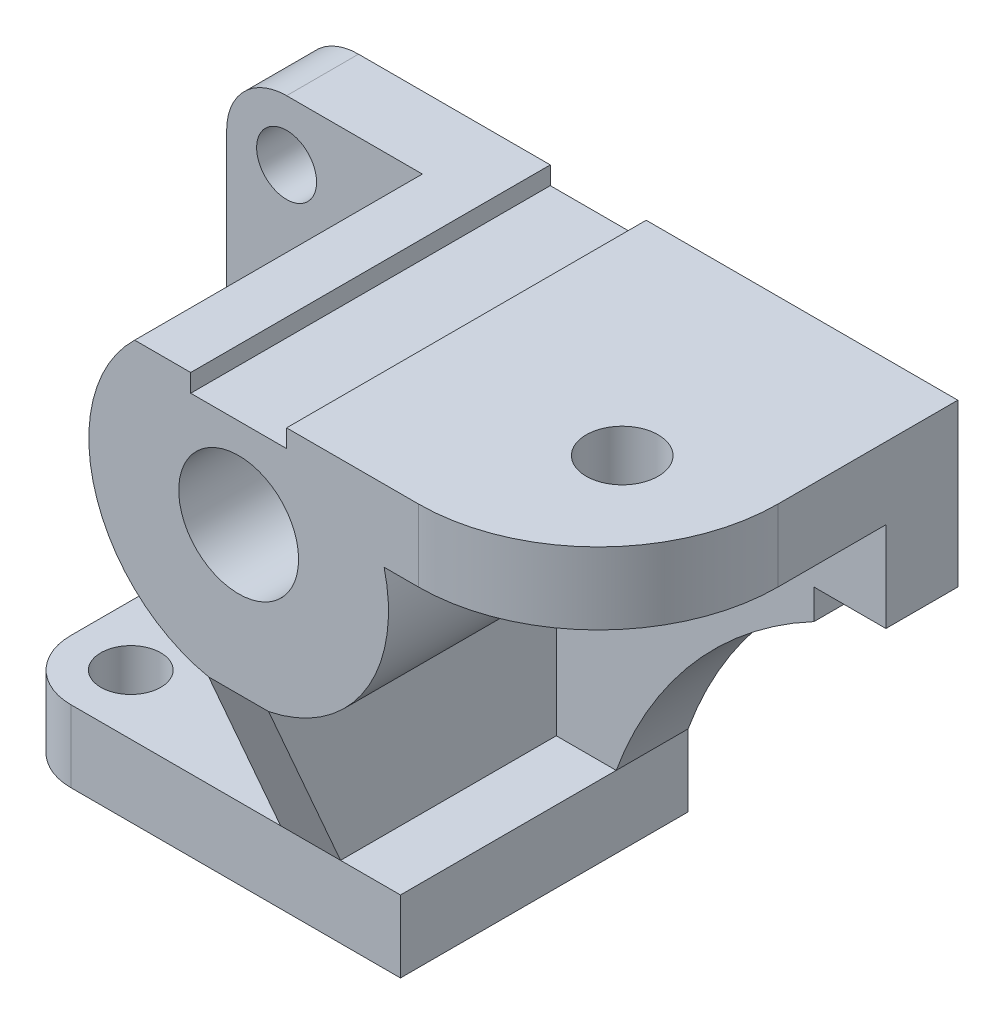
ISO-10303-21;
HEADER;
FILE_DESCRIPTION(('STEP AP214'),'2;1');
FILE_NAME('part.step','',(''),(''),'','','');
FILE_SCHEMA(('AUTOMOTIVE_DESIGN { 1 0 10303 214 1 1 1 1 }'));
ENDSEC;
DATA;
#1=APPLICATION_CONTEXT('core data for automotive mechanical design processes');
#2=APPLICATION_PROTOCOL_DEFINITION('international standard','automotive_design',2000,#1);
#3=PRODUCT_CONTEXT('',#1,'mechanical');
#4=PRODUCT('Part','Part','',(#3));
#5=PRODUCT_RELATED_PRODUCT_CATEGORY('part','',(#4));
#6=PRODUCT_DEFINITION_FORMATION('','',#4);
#7=PRODUCT_DEFINITION_CONTEXT('part definition',#1,'design');
#8=PRODUCT_DEFINITION('design','',#6,#7);
#9=PRODUCT_DEFINITION_SHAPE('','',#8);
#10=(LENGTH_UNIT() NAMED_UNIT(*) SI_UNIT(.MILLI.,.METRE.));
#11=(NAMED_UNIT(*) PLANE_ANGLE_UNIT() SI_UNIT($,.RADIAN.));
#12=(NAMED_UNIT(*) SI_UNIT($,.STERADIAN.) SOLID_ANGLE_UNIT());
#13=UNCERTAINTY_MEASURE_WITH_UNIT(LENGTH_MEASURE(1.E-05),#10,'distance_accuracy_value','');
#14=(GEOMETRIC_REPRESENTATION_CONTEXT(3) GLOBAL_UNCERTAINTY_ASSIGNED_CONTEXT((#13)) GLOBAL_UNIT_ASSIGNED_CONTEXT((#10,
#11,#12)) REPRESENTATION_CONTEXT('',''));
#15=CARTESIAN_POINT('',(0.,0.,0.));
#16=DIRECTION('',(0.,0.,1.));
#17=DIRECTION('',(1.,0.,0.));
#18=AXIS2_PLACEMENT_3D('',#15,#16,#17);
#19=CARTESIAN_POINT('',(98.3190383965627,-11.8296912391202,-12.));
#20=DIRECTION('',(0.,0.,1.));
#21=DIRECTION('',(1.,0.,0.));
#22=AXIS2_PLACEMENT_3D('',#19,#20,#21);
#23=PLANE('',#22);
#24=CARTESIAN_POINT('',(17.5,64.,-12.));
#25=DIRECTION('',(0.,0.,1.));
#26=DIRECTION('',(1.,0.,0.));
#27=AXIS2_PLACEMENT_3D('',#24,#25,#26);
#28=CIRCLE('',#27,25.);
#29=CARTESIAN_POINT('',(22.5,39.5051025721682,-12.));
#30=VERTEX_POINT('',#29);
#31=CARTESIAN_POINT('',(41.7693221990232,70.,-12.));
#32=VERTEX_POINT('',#31);
#33=EDGE_CURVE('E344',#30,#32,#28,.T.);
#34=ORIENTED_EDGE('',*,*,#33,.F.);
#35=DIRECTION('',(0.,1.,0.));
#36=VECTOR('',#35,1.);
#37=CARTESIAN_POINT('',(22.5,39.5051025721682,-12.));
#38=LINE('',#37,#36);
#39=CARTESIAN_POINT('',(22.5,12.,-12.));
#40=VERTEX_POINT('',#39);
#41=EDGE_CURVE('E428',#40,#30,#38,.T.);
#42=ORIENTED_EDGE('',*,*,#41,.F.);
#43=DIRECTION('',(-1.,0.,0.));
#44=VECTOR('',#43,1.);
#45=CARTESIAN_POINT('',(32.5,12.,-12.));
#46=LINE('',#45,#44);
#47=CARTESIAN_POINT('',(32.5,12.,-12.));
#48=VERTEX_POINT('',#47);
#49=EDGE_CURVE('E233',#48,#40,#46,.T.);
#50=ORIENTED_EDGE('',*,*,#49,.F.);
#51=CARTESIAN_POINT('',(98.3190383965627,-11.8296912391202,-12.));
#52=DIRECTION('',(0.,0.,1.));
#53=DIRECTION('',(1.,0.,0.));
#54=AXIS2_PLACEMENT_3D('',#51,#52,#53);
#55=CIRCLE('',#54,70.);
#56=CARTESIAN_POINT('',(65.5,50.,-12.));
#57=VERTEX_POINT('',#56);
#58=EDGE_CURVE('E377',#57,#48,#55,.T.);
#59=ORIENTED_EDGE('',*,*,#58,.F.);
#60=DIRECTION('',(0.,-1.,0.));
#61=VECTOR('',#60,1.);
#62=CARTESIAN_POINT('',(65.5,55.,-12.));
#63=LINE('',#62,#61);
#64=CARTESIAN_POINT('',(65.5,55.,-12.));
#65=VERTEX_POINT('',#64);
#66=EDGE_CURVE('E374',#65,#57,#63,.T.);
#67=ORIENTED_EDGE('',*,*,#66,.F.);
#68=DIRECTION('',(-1.,0.,0.));
#69=VECTOR('',#68,1.);
#70=CARTESIAN_POINT('',(77.5,55.,-12.));
#71=LINE('',#70,#69);
#72=CARTESIAN_POINT('',(77.5,55.,-12.));
#73=VERTEX_POINT('',#72);
#74=EDGE_CURVE('E375',#73,#65,#71,.T.);
#75=ORIENTED_EDGE('',*,*,#74,.F.);
#76=DIRECTION('',(0.,-1.,0.));
#77=VECTOR('',#76,1.);
#78=CARTESIAN_POINT('',(77.5,82.,-12.));
#79=LINE('',#78,#77);
#80=CARTESIAN_POINT('',(77.5,70.,-12.));
#81=VERTEX_POINT('',#80);
#82=EDGE_CURVE('E369',#81,#73,#79,.T.);
#83=ORIENTED_EDGE('',*,*,#82,.F.);
#84=DIRECTION('',(-1.,0.,0.));
#85=VECTOR('',#84,1.);
#86=CARTESIAN_POINT('',(98.3190383965627,70.,-12.));
#87=LINE('',#86,#85);
#88=EDGE_CURVE('E463',#81,#32,#87,.T.);
#89=ORIENTED_EDGE('',*,*,#88,.T.);
#90=EDGE_LOOP('',(#34,#42,#50,#59,#67,#75,#83,#89));
#91=FACE_BOUND('',#90,.T.);
#92=ADVANCED_FACE('F44',(#91),#23,.T.);
#93=CARTESIAN_POINT('',(-22.5,72.,-12.));
#94=DIRECTION('',(0.,0.,1.));
#95=DIRECTION('',(1.,0.,0.));
#96=AXIS2_PLACEMENT_3D('',#93,#94,#95);
#97=CIRCLE('',#96,5.);
#98=CARTESIAN_POINT('',(-17.5,72.,-12.));
#99=VERTEX_POINT('',#98);
#100=EDGE_CURVE('E441',#99,#99,#97,.T.);
#101=ORIENTED_EDGE('',*,*,#100,.F.);
#102=EDGE_LOOP('',(#101));
#103=FACE_BOUND('',#102,.T.);
#104=CARTESIAN_POINT('',(12.5,12.,-12.));
#105=VERTEX_POINT('',#104);
#106=CARTESIAN_POINT('',(-32.5,12.,-12.));
#107=VERTEX_POINT('',#106);
#108=EDGE_CURVE('E370',#105,#107,#46,.T.);
#109=ORIENTED_EDGE('',*,*,#108,.F.);
#110=DIRECTION('',(0.,-1.,0.));
#111=VECTOR('',#110,1.);
#112=CARTESIAN_POINT('',(12.5,12.,-12.));
#113=LINE('',#112,#111);
#114=CARTESIAN_POINT('',(12.5,39.5051025721682,-12.));
#115=VERTEX_POINT('',#114);
#116=EDGE_CURVE('E426',#115,#105,#113,.T.);
#117=ORIENTED_EDGE('',*,*,#116,.F.);
#118=CARTESIAN_POINT('',(0.150648427102509,82.,-12.));
#119=VERTEX_POINT('',#118);
#120=EDGE_CURVE('E349',#119,#115,#28,.T.);
#121=ORIENTED_EDGE('',*,*,#120,.F.);
#122=DIRECTION('',(1.,0.,0.));
#123=VECTOR('',#122,1.);
#124=CARTESIAN_POINT('',(-32.5,82.,-12.));
#125=LINE('',#124,#123);
#126=CARTESIAN_POINT('',(-22.5,82.,-12.));
#127=VERTEX_POINT('',#126);
#128=EDGE_CURVE('E292',#127,#119,#125,.T.);
#129=ORIENTED_EDGE('',*,*,#128,.F.);
#130=CARTESIAN_POINT('',(-22.5,72.,-12.));
#131=DIRECTION('',(0.,0.,1.));
#132=DIRECTION('',(1.,0.,0.));
#133=AXIS2_PLACEMENT_3D('',#130,#131,#132);
#134=CIRCLE('',#133,10.);
#135=CARTESIAN_POINT('',(-32.5,72.,-12.));
#136=VERTEX_POINT('',#135);
#137=EDGE_CURVE('E52',#127,#136,#134,.T.);
#138=ORIENTED_EDGE('',*,*,#137,.T.);
#139=DIRECTION('',(0.,1.,0.));
#140=VECTOR('',#139,1.);
#141=CARTESIAN_POINT('',(-32.5,12.,-12.));
#142=LINE('',#141,#140);
#143=EDGE_CURVE('E287',#107,#136,#142,.T.);
#144=ORIENTED_EDGE('',*,*,#143,.F.);
#145=EDGE_LOOP('',(#109,#117,#121,#129,#138,#144));
#146=FACE_BOUND('',#145,.T.);
#147=ADVANCED_FACE('F288',(#103,#146),#23,.T.);
#148=CARTESIAN_POINT('',(17.5,64.,36.));
#149=DIRECTION('',(0.,0.,-1.));
#150=DIRECTION('',(-1.,0.,0.));
#151=AXIS2_PLACEMENT_3D('',#148,#149,#150);
#152=CYLINDRICAL_SURFACE('',#151,25.);
#153=DIRECTION('',(0.,0.,-1.));
#154=VECTOR('',#153,1.);
#155=CARTESIAN_POINT('',(22.5,39.5051025721682,36.));
#156=LINE('',#155,#154);
#157=CARTESIAN_POINT('',(22.5,39.5051025721682,36.));
#158=VERTEX_POINT('',#157);
#159=EDGE_CURVE('E225',#158,#30,#156,.T.);
#160=ORIENTED_EDGE('',*,*,#159,.T.);
#161=ORIENTED_EDGE('',*,*,#33,.T.);
#162=DIRECTION('',(0.,0.,-1.));
#163=VECTOR('',#162,1.);
#164=CARTESIAN_POINT('',(41.7693221990232,70.,36.));
#165=LINE('',#164,#163);
#166=CARTESIAN_POINT('',(41.7693221990232,70.,36.));
#167=VERTEX_POINT('',#166);
#168=EDGE_CURVE('E457',#167,#32,#165,.T.);
#169=ORIENTED_EDGE('',*,*,#168,.F.);
#170=CARTESIAN_POINT('',(17.5,64.,36.));
#171=DIRECTION('',(0.,0.,1.));
#172=DIRECTION('',(1.,0.,0.));
#173=AXIS2_PLACEMENT_3D('',#170,#171,#172);
#174=CIRCLE('',#173,25.);
#175=EDGE_CURVE('E360',#158,#167,#174,.T.);
#176=ORIENTED_EDGE('',*,*,#175,.F.);
#177=EDGE_LOOP('',(#160,#161,#169,#176));
#178=FACE_BOUND('',#177,.T.);
#179=ADVANCED_FACE('F317',(#178),#152,.T.);
#180=DIRECTION('',(0.,0.,-1.));
#181=VECTOR('',#180,1.);
#182=CARTESIAN_POINT('',(12.5,39.5051025721682,36.));
#183=LINE('',#182,#181);
#184=CARTESIAN_POINT('',(12.5,39.5051025721682,36.));
#185=VERTEX_POINT('',#184);
#186=EDGE_CURVE('E434',#185,#115,#183,.T.);
#187=ORIENTED_EDGE('',*,*,#186,.F.);
#188=CARTESIAN_POINT('',(0.150648427102509,82.,36.));
#189=VERTEX_POINT('',#188);
#190=EDGE_CURVE('E354',#189,#185,#174,.T.);
#191=ORIENTED_EDGE('',*,*,#190,.F.);
#192=DIRECTION('',(0.,0.,-1.));
#193=VECTOR('',#192,1.);
#194=CARTESIAN_POINT('',(0.150648427102509,82.,36.));
#195=LINE('',#194,#193);
#196=EDGE_CURVE('E363',#189,#119,#195,.T.);
#197=ORIENTED_EDGE('',*,*,#196,.T.);
#198=ORIENTED_EDGE('',*,*,#120,.T.);
#199=EDGE_LOOP('',(#187,#191,#197,#198));
#200=FACE_BOUND('',#199,.T.);
#201=ADVANCED_FACE('F500',(#200),#152,.T.);
#202=CARTESIAN_POINT('',(0.,12.,0.));
#203=DIRECTION('',(0.,-1.,0.));
#204=DIRECTION('',(0.,0.,-1.));
#205=AXIS2_PLACEMENT_3D('',#202,#203,#204);
#206=PLANE('',#205);
#207=DIRECTION('',(0.,0.,-1.));
#208=VECTOR('',#207,1.);
#209=CARTESIAN_POINT('',(22.5,12.,36.));
#210=LINE('',#209,#208);
#211=CARTESIAN_POINT('',(22.5,12.,24.));
#212=VERTEX_POINT('',#211);
#213=EDGE_CURVE('E218',#212,#40,#210,.T.);
#214=ORIENTED_EDGE('',*,*,#213,.F.);
#215=DIRECTION('',(1.,0.,0.));
#216=VECTOR('',#215,1.);
#217=CARTESIAN_POINT('',(-32.5,12.,24.));
#218=LINE('',#217,#216);
#219=CARTESIAN_POINT('',(32.5,12.,24.));
#220=VERTEX_POINT('',#219);
#221=EDGE_CURVE('E214',#212,#220,#218,.T.);
#222=ORIENTED_EDGE('',*,*,#221,.T.);
#223=DIRECTION('',(0.,0.,-1.));
#224=VECTOR('',#223,1.);
#225=CARTESIAN_POINT('',(32.5,12.,24.));
#226=LINE('',#225,#224);
#227=EDGE_CURVE('E239',#220,#48,#226,.T.);
#228=ORIENTED_EDGE('',*,*,#227,.T.);
#229=ORIENTED_EDGE('',*,*,#49,.T.);
#230=EDGE_LOOP('',(#214,#222,#228,#229));
#231=FACE_BOUND('',#230,.T.);
#232=ADVANCED_FACE('F226',(#231),#206,.F.);
#233=CARTESIAN_POINT('',(-22.5,12.,14.));
#234=DIRECTION('',(0.,1.,0.));
#235=DIRECTION('',(0.,0.,1.));
#236=AXIS2_PLACEMENT_3D('',#233,#234,#235);
#237=CIRCLE('',#236,5.);
#238=CARTESIAN_POINT('',(-22.5,12.,19.));
#239=VERTEX_POINT('',#238);
#240=EDGE_CURVE('E235',#239,#239,#237,.T.);
#241=ORIENTED_EDGE('',*,*,#240,.F.);
#242=EDGE_LOOP('',(#241));
#243=FACE_BOUND('',#242,.T.);
#244=DIRECTION('',(0.,0.,-1.));
#245=VECTOR('',#244,1.);
#246=CARTESIAN_POINT('',(12.5,12.,36.));
#247=LINE('',#246,#245);
#248=CARTESIAN_POINT('',(12.5,12.,24.));
#249=VERTEX_POINT('',#248);
#250=EDGE_CURVE('E427',#249,#105,#247,.T.);
#251=ORIENTED_EDGE('',*,*,#250,.T.);
#252=ORIENTED_EDGE('',*,*,#108,.T.);
#253=DIRECTION('',(0.,0.,1.));
#254=VECTOR('',#253,1.);
#255=CARTESIAN_POINT('',(-32.5,12.,24.));
#256=LINE('',#255,#254);
#257=CARTESIAN_POINT('',(-32.5,12.,14.));
#258=VERTEX_POINT('',#257);
#259=EDGE_CURVE('E238',#107,#258,#256,.T.);
#260=ORIENTED_EDGE('',*,*,#259,.T.);
#261=CARTESIAN_POINT('',(-22.5,12.,14.));
#262=DIRECTION('',(0.,-1.,0.));
#263=DIRECTION('',(0.,0.,-1.));
#264=AXIS2_PLACEMENT_3D('',#261,#262,#263);
#265=CIRCLE('',#264,10.);
#266=CARTESIAN_POINT('',(-22.5,12.,24.));
#267=VERTEX_POINT('',#266);
#268=EDGE_CURVE('E278',#258,#267,#265,.F.);
#269=ORIENTED_EDGE('',*,*,#268,.T.);
#270=EDGE_CURVE('E215',#267,#249,#218,.T.);
#271=ORIENTED_EDGE('',*,*,#270,.T.);
#272=EDGE_LOOP('',(#251,#252,#260,#269,#271));
#273=FACE_BOUND('',#272,.T.);
#274=ADVANCED_FACE('F501',(#243,#273),#206,.F.);
#275=CARTESIAN_POINT('',(-32.5,82.,-12.));
#276=DIRECTION('',(0.,1.,0.));
#277=DIRECTION('',(0.,0.,1.));
#278=AXIS2_PLACEMENT_3D('',#275,#276,#277);
#279=PLANE('',#278);
#280=DIRECTION('',(1.,0.,0.));
#281=VECTOR('',#280,1.);
#282=CARTESIAN_POINT('',(-32.5,82.,-24.));
#283=LINE('',#282,#281);
#284=CARTESIAN_POINT('',(-22.5,82.,-24.));
#285=VERTEX_POINT('',#284);
#286=CARTESIAN_POINT('',(9.49999999999999,82.,-24.));
#287=VERTEX_POINT('',#286);
#288=EDGE_CURVE('E385',#285,#287,#283,.T.);
#289=ORIENTED_EDGE('',*,*,#288,.F.);
#290=DIRECTION('',(0.,0.,-1.));
#291=VECTOR('',#290,1.);
#292=CARTESIAN_POINT('',(-22.5,82.,-12.));
#293=LINE('',#292,#291);
#294=EDGE_CURVE('E58',#285,#127,#293,.F.);
#295=ORIENTED_EDGE('',*,*,#294,.T.);
#296=ORIENTED_EDGE('',*,*,#128,.T.);
#297=ORIENTED_EDGE('',*,*,#196,.F.);
#298=DIRECTION('',(-1.,0.,0.));
#299=VECTOR('',#298,1.);
#300=CARTESIAN_POINT('',(0.150648427102509,82.,36.));
#301=LINE('',#300,#299);
#302=CARTESIAN_POINT('',(9.49999999999999,82.,36.));
#303=VERTEX_POINT('',#302);
#304=EDGE_CURVE('E356',#303,#189,#301,.T.);
#305=ORIENTED_EDGE('',*,*,#304,.F.);
#306=DIRECTION('',(0.,0.,1.));
#307=VECTOR('',#306,1.);
#308=CARTESIAN_POINT('',(9.49999999999999,82.,-24.));
#309=LINE('',#308,#307);
#310=EDGE_CURVE('E464',#287,#303,#309,.T.);
#311=ORIENTED_EDGE('',*,*,#310,.F.);
#312=EDGE_LOOP('',(#289,#295,#296,#297,#305,#311));
#313=FACE_BOUND('',#312,.T.);
#314=ADVANCED_FACE('F491',(#313),#279,.T.);
#315=CARTESIAN_POINT('',(32.5,12.,24.));
#316=DIRECTION('',(-1.,0.,0.));
#317=DIRECTION('',(0.,0.,1.));
#318=AXIS2_PLACEMENT_3D('',#315,#316,#317);
#319=PLANE('',#318);
#320=DIRECTION('',(0.,0.,-1.));
#321=VECTOR('',#320,1.);
#322=CARTESIAN_POINT('',(32.5,0.,24.));
#323=LINE('',#322,#321);
#324=CARTESIAN_POINT('',(32.5,0.,24.));
#325=VERTEX_POINT('',#324);
#326=CARTESIAN_POINT('',(32.5,0.,-24.));
#327=VERTEX_POINT('',#326);
#328=EDGE_CURVE('E400',#325,#327,#323,.T.);
#329=ORIENTED_EDGE('',*,*,#328,.T.);
#330=DIRECTION('',(0.,-1.,0.));
#331=VECTOR('',#330,1.);
#332=CARTESIAN_POINT('',(32.5,12.,-24.));
#333=LINE('',#332,#331);
#334=CARTESIAN_POINT('',(32.5,12.,-24.));
#335=VERTEX_POINT('',#334);
#336=EDGE_CURVE('E249',#335,#327,#333,.T.);
#337=ORIENTED_EDGE('',*,*,#336,.F.);
#338=DIRECTION('',(0.,0.,-1.));
#339=VECTOR('',#338,1.);
#340=CARTESIAN_POINT('',(32.5,12.,-12.));
#341=LINE('',#340,#339);
#342=EDGE_CURVE('E392',#48,#335,#341,.T.);
#343=ORIENTED_EDGE('',*,*,#342,.F.);
#344=ORIENTED_EDGE('',*,*,#227,.F.);
#345=DIRECTION('',(0.,-1.,0.));
#346=VECTOR('',#345,1.);
#347=CARTESIAN_POINT('',(32.5,12.,24.));
#348=LINE('',#347,#346);
#349=EDGE_CURVE('E236',#220,#325,#348,.T.);
#350=ORIENTED_EDGE('',*,*,#349,.T.);
#351=EDGE_LOOP('',(#329,#337,#343,#344,#350));
#352=FACE_BOUND('',#351,.T.);
#353=ADVANCED_FACE('F413',(#352),#319,.F.);
#354=CARTESIAN_POINT('',(-32.5,12.,-24.));
#355=DIRECTION('',(0.,0.,1.));
#356=DIRECTION('',(1.,0.,0.));
#357=AXIS2_PLACEMENT_3D('',#354,#355,#356);
#358=PLANE('',#357);
#359=CARTESIAN_POINT('',(-22.5,72.,-24.));
#360=DIRECTION('',(0.,0.,1.));
#361=DIRECTION('',(1.,0.,0.));
#362=AXIS2_PLACEMENT_3D('',#359,#360,#361);
#363=CIRCLE('',#362,5.);
#364=CARTESIAN_POINT('',(-17.5,72.,-24.));
#365=VERTEX_POINT('',#364);
#366=EDGE_CURVE('E443',#365,#365,#363,.T.);
#367=ORIENTED_EDGE('',*,*,#366,.T.);
#368=EDGE_LOOP('',(#367));
#369=FACE_BOUND('',#368,.T.);
#370=DIRECTION('',(0.,-1.,0.));
#371=VECTOR('',#370,1.);
#372=CARTESIAN_POINT('',(-32.5,12.,-24.));
#373=LINE('',#372,#371);
#374=CARTESIAN_POINT('',(-32.5,72.,-24.));
#375=VERTEX_POINT('',#374);
#376=CARTESIAN_POINT('',(-32.5,0.,-24.));
#377=VERTEX_POINT('',#376);
#378=EDGE_CURVE('E244',#375,#377,#373,.T.);
#379=ORIENTED_EDGE('',*,*,#378,.F.);
#380=CARTESIAN_POINT('',(-22.5,72.,-24.));
#381=DIRECTION('',(0.,0.,1.));
#382=DIRECTION('',(1.,0.,0.));
#383=AXIS2_PLACEMENT_3D('',#380,#381,#382);
#384=CIRCLE('',#383,10.);
#385=EDGE_CURVE('E70',#375,#285,#384,.F.);
#386=ORIENTED_EDGE('',*,*,#385,.T.);
#387=ORIENTED_EDGE('',*,*,#288,.T.);
#388=DIRECTION('',(0.,1.,0.));
#389=VECTOR('',#388,1.);
#390=CARTESIAN_POINT('',(9.49999999999999,79.,-24.));
#391=LINE('',#390,#389);
#392=CARTESIAN_POINT('',(9.49999999999999,79.,-24.));
#393=VERTEX_POINT('',#392);
#394=EDGE_CURVE('E341',#393,#287,#391,.T.);
#395=ORIENTED_EDGE('',*,*,#394,.F.);
#396=DIRECTION('',(-1.,0.,0.));
#397=VECTOR('',#396,1.);
#398=CARTESIAN_POINT('',(9.49999999999999,79.,-24.));
#399=LINE('',#398,#397);
#400=CARTESIAN_POINT('',(25.5,79.,-24.));
#401=VERTEX_POINT('',#400);
#402=EDGE_CURVE('E473',#401,#393,#399,.T.);
#403=ORIENTED_EDGE('',*,*,#402,.F.);
#404=DIRECTION('',(0.,1.,0.));
#405=VECTOR('',#404,1.);
#406=CARTESIAN_POINT('',(25.5,79.,-24.));
#407=LINE('',#406,#405);
#408=CARTESIAN_POINT('',(25.5,82.,-24.));
#409=VERTEX_POINT('',#408);
#410=EDGE_CURVE('E348',#401,#409,#407,.T.);
#411=ORIENTED_EDGE('',*,*,#410,.T.);
#412=CARTESIAN_POINT('',(77.5,82.,-24.));
#413=VERTEX_POINT('',#412);
#414=EDGE_CURVE('E366',#409,#413,#283,.T.);
#415=ORIENTED_EDGE('',*,*,#414,.T.);
#416=DIRECTION('',(0.,-1.,0.));
#417=VECTOR('',#416,1.);
#418=CARTESIAN_POINT('',(77.5,82.,-24.));
#419=LINE('',#418,#417);
#420=CARTESIAN_POINT('',(77.5,55.,-24.));
#421=VERTEX_POINT('',#420);
#422=EDGE_CURVE('E381',#413,#421,#419,.T.);
#423=ORIENTED_EDGE('',*,*,#422,.T.);
#424=DIRECTION('',(-1.,0.,0.));
#425=VECTOR('',#424,1.);
#426=CARTESIAN_POINT('',(77.5,55.,-24.));
#427=LINE('',#426,#425);
#428=CARTESIAN_POINT('',(65.5,55.,-24.));
#429=VERTEX_POINT('',#428);
#430=EDGE_CURVE('E387',#421,#429,#427,.T.);
#431=ORIENTED_EDGE('',*,*,#430,.T.);
#432=DIRECTION('',(0.,-1.,0.));
#433=VECTOR('',#432,1.);
#434=CARTESIAN_POINT('',(65.5,55.,-24.));
#435=LINE('',#434,#433);
#436=CARTESIAN_POINT('',(65.5,50.,-24.));
#437=VERTEX_POINT('',#436);
#438=EDGE_CURVE('E386',#429,#437,#435,.T.);
#439=ORIENTED_EDGE('',*,*,#438,.T.);
#440=CARTESIAN_POINT('',(98.3190383965627,-11.8296912391202,-24.));
#441=DIRECTION('',(0.,0.,1.));
#442=DIRECTION('',(1.,0.,0.));
#443=AXIS2_PLACEMENT_3D('',#440,#441,#442);
#444=CIRCLE('',#443,70.);
#445=EDGE_CURVE('E391',#437,#335,#444,.T.);
#446=ORIENTED_EDGE('',*,*,#445,.T.);
#447=ORIENTED_EDGE('',*,*,#336,.T.);
#448=DIRECTION('',(-1.,0.,0.));
#449=VECTOR('',#448,1.);
#450=CARTESIAN_POINT('',(-32.5,0.,-24.));
#451=LINE('',#450,#449);
#452=EDGE_CURVE('E409',#327,#377,#451,.T.);
#453=ORIENTED_EDGE('',*,*,#452,.T.);
#454=EDGE_LOOP('',(#379,#386,#387,#395,#403,#411,#415,#423,#431,#439,#446,#447,#453));
#455=FACE_BOUND('',#454,.T.);
#456=ADVANCED_FACE('F418',(#369,#455),#358,.F.);
#457=CARTESIAN_POINT('',(-32.5,12.,24.));
#458=DIRECTION('',(1.,0.,0.));
#459=DIRECTION('',(0.,0.,-1.));
#460=AXIS2_PLACEMENT_3D('',#457,#458,#459);
#461=PLANE('',#460);
#462=DIRECTION('',(0.,0.,1.));
#463=VECTOR('',#462,1.);
#464=CARTESIAN_POINT('',(-32.5,0.,24.));
#465=LINE('',#464,#463);
#466=CARTESIAN_POINT('',(-32.5,0.,14.));
#467=VERTEX_POINT('',#466);
#468=EDGE_CURVE('E407',#377,#467,#465,.T.);
#469=ORIENTED_EDGE('',*,*,#468,.T.);
#470=DIRECTION('',(0.,-1.,0.));
#471=VECTOR('',#470,1.);
#472=CARTESIAN_POINT('',(-32.5,12.,14.));
#473=LINE('',#472,#471);
#474=EDGE_CURVE('E279',#467,#258,#473,.F.);
#475=ORIENTED_EDGE('',*,*,#474,.T.);
#476=ORIENTED_EDGE('',*,*,#259,.F.);
#477=ORIENTED_EDGE('',*,*,#143,.T.);
#478=DIRECTION('',(0.,0.,-1.));
#479=VECTOR('',#478,1.);
#480=CARTESIAN_POINT('',(-32.5,72.,-24.));
#481=LINE('',#480,#479);
#482=EDGE_CURVE('E273',#136,#375,#481,.T.);
#483=ORIENTED_EDGE('',*,*,#482,.T.);
#484=ORIENTED_EDGE('',*,*,#378,.T.);
#485=EDGE_LOOP('',(#469,#475,#476,#477,#483,#484));
#486=FACE_BOUND('',#485,.T.);
#487=ADVANCED_FACE('F300',(#486),#461,.F.);
#488=CARTESIAN_POINT('',(-32.5,12.,24.));
#489=DIRECTION('',(0.,0.,-1.));
#490=DIRECTION('',(-1.,0.,0.));
#491=AXIS2_PLACEMENT_3D('',#488,#489,#490);
#492=PLANE('',#491);
#493=ORIENTED_EDGE('',*,*,#270,.F.);
#494=DIRECTION('',(0.,-1.,0.));
#495=VECTOR('',#494,1.);
#496=CARTESIAN_POINT('',(-22.5,12.,24.));
#497=LINE('',#496,#495);
#498=CARTESIAN_POINT('',(-22.5,0.,24.));
#499=VERTEX_POINT('',#498);
#500=EDGE_CURVE('E269',#267,#499,#497,.T.);
#501=ORIENTED_EDGE('',*,*,#500,.T.);
#502=DIRECTION('',(1.,0.,0.));
#503=VECTOR('',#502,1.);
#504=CARTESIAN_POINT('',(-32.5,0.,24.));
#505=LINE('',#504,#503);
#506=EDGE_CURVE('E254',#499,#325,#505,.T.);
#507=ORIENTED_EDGE('',*,*,#506,.T.);
#508=ORIENTED_EDGE('',*,*,#349,.F.);
#509=ORIENTED_EDGE('',*,*,#221,.F.);
#510=EDGE_CURVE('E205',#249,#212,#218,.T.);
#511=ORIENTED_EDGE('',*,*,#510,.F.);
#512=EDGE_LOOP('',(#493,#501,#507,#508,#509,#511));
#513=FACE_BOUND('',#512,.T.);
#514=ADVANCED_FACE('F234',(#513),#492,.F.);
#515=CARTESIAN_POINT('',(0.,0.,0.));
#516=DIRECTION('',(0.,-1.,0.));
#517=DIRECTION('',(0.,0.,-1.));
#518=AXIS2_PLACEMENT_3D('',#515,#516,#517);
#519=PLANE('',#518);
#520=CARTESIAN_POINT('',(-22.5,0.,14.));
#521=DIRECTION('',(0.,1.,0.));
#522=DIRECTION('',(0.,0.,1.));
#523=AXIS2_PLACEMENT_3D('',#520,#521,#522);
#524=CIRCLE('',#523,5.);
#525=CARTESIAN_POINT('',(-22.5,0.,19.));
#526=VERTEX_POINT('',#525);
#527=EDGE_CURVE('E438',#526,#526,#524,.T.);
#528=ORIENTED_EDGE('',*,*,#527,.T.);
#529=EDGE_LOOP('',(#528));
#530=FACE_BOUND('',#529,.T.);
#531=ORIENTED_EDGE('',*,*,#506,.F.);
#532=CARTESIAN_POINT('',(-22.5,0.,14.));
#533=DIRECTION('',(0.,-1.,0.));
#534=DIRECTION('',(0.,0.,-1.));
#535=AXIS2_PLACEMENT_3D('',#532,#533,#534);
#536=CIRCLE('',#535,10.);
#537=EDGE_CURVE('E271',#499,#467,#536,.T.);
#538=ORIENTED_EDGE('',*,*,#537,.T.);
#539=ORIENTED_EDGE('',*,*,#468,.F.);
#540=ORIENTED_EDGE('',*,*,#452,.F.);
#541=ORIENTED_EDGE('',*,*,#328,.F.);
#542=EDGE_LOOP('',(#531,#538,#539,#540,#541));
#543=FACE_BOUND('',#542,.T.);
#544=ADVANCED_FACE('F420',(#530,#543),#519,.T.);
#545=CARTESIAN_POINT('',(98.3190383965627,-11.8296912391202,-12.));
#546=DIRECTION('',(0.,0.,-1.));
#547=DIRECTION('',(-1.,0.,0.));
#548=AXIS2_PLACEMENT_3D('',#545,#546,#547);
#549=CYLINDRICAL_SURFACE('',#548,70.);
#550=ORIENTED_EDGE('',*,*,#445,.F.);
#551=DIRECTION('',(0.,0.,-1.));
#552=VECTOR('',#551,1.);
#553=CARTESIAN_POINT('',(65.5,50.,-12.));
#554=LINE('',#553,#552);
#555=EDGE_CURVE('E398',#57,#437,#554,.T.);
#556=ORIENTED_EDGE('',*,*,#555,.F.);
#557=ORIENTED_EDGE('',*,*,#58,.T.);
#558=ORIENTED_EDGE('',*,*,#342,.T.);
#559=EDGE_LOOP('',(#550,#556,#557,#558));
#560=FACE_BOUND('',#559,.T.);
#561=ADVANCED_FACE('F422',(#560),#549,.F.);
#562=CARTESIAN_POINT('',(65.5,55.,-12.));
#563=DIRECTION('',(1.,0.,0.));
#564=DIRECTION('',(0.,0.,-1.));
#565=AXIS2_PLACEMENT_3D('',#562,#563,#564);
#566=PLANE('',#565);
#567=ORIENTED_EDGE('',*,*,#438,.F.);
#568=DIRECTION('',(0.,0.,-1.));
#569=VECTOR('',#568,1.);
#570=CARTESIAN_POINT('',(65.5,55.,-12.));
#571=LINE('',#570,#569);
#572=EDGE_CURVE('E399',#65,#429,#571,.T.);
#573=ORIENTED_EDGE('',*,*,#572,.F.);
#574=ORIENTED_EDGE('',*,*,#66,.T.);
#575=ORIENTED_EDGE('',*,*,#555,.T.);
#576=EDGE_LOOP('',(#567,#573,#574,#575));
#577=FACE_BOUND('',#576,.T.);
#578=ADVANCED_FACE('F583',(#577),#566,.T.);
#579=CARTESIAN_POINT('',(77.5,55.,-12.));
#580=DIRECTION('',(0.,-1.,0.));
#581=DIRECTION('',(0.,0.,-1.));
#582=AXIS2_PLACEMENT_3D('',#579,#580,#581);
#583=PLANE('',#582);
#584=ORIENTED_EDGE('',*,*,#430,.F.);
#585=DIRECTION('',(0.,0.,-1.));
#586=VECTOR('',#585,1.);
#587=CARTESIAN_POINT('',(77.5,55.,-12.));
#588=LINE('',#587,#586);
#589=EDGE_CURVE('E405',#73,#421,#588,.T.);
#590=ORIENTED_EDGE('',*,*,#589,.F.);
#591=ORIENTED_EDGE('',*,*,#74,.T.);
#592=ORIENTED_EDGE('',*,*,#572,.T.);
#593=EDGE_LOOP('',(#584,#590,#591,#592));
#594=FACE_BOUND('',#593,.T.);
#595=ADVANCED_FACE('F584',(#594),#583,.T.);
#596=CARTESIAN_POINT('',(77.5,82.,-12.));
#597=DIRECTION('',(1.,0.,0.));
#598=DIRECTION('',(0.,0.,-1.));
#599=AXIS2_PLACEMENT_3D('',#596,#597,#598);
#600=PLANE('',#599);
#601=DIRECTION('',(0.,0.,-1.));
#602=VECTOR('',#601,1.);
#603=CARTESIAN_POINT('',(77.5,82.,-12.));
#604=LINE('',#603,#602);
#605=CARTESIAN_POINT('',(77.5,82.,6.00000000000001));
#606=VERTEX_POINT('',#605);
#607=EDGE_CURVE('E382',#606,#413,#604,.T.);
#608=ORIENTED_EDGE('',*,*,#607,.F.);
#609=DIRECTION('',(0.,1.,0.));
#610=VECTOR('',#609,1.);
#611=CARTESIAN_POINT('',(77.5,82.,6.00000000000001));
#612=LINE('',#611,#610);
#613=CARTESIAN_POINT('',(77.5,70.,6.00000000000001));
#614=VERTEX_POINT('',#613);
#615=EDGE_CURVE('E266',#606,#614,#612,.F.);
#616=ORIENTED_EDGE('',*,*,#615,.T.);
#617=DIRECTION('',(0.,0.,-1.));
#618=VECTOR('',#617,1.);
#619=CARTESIAN_POINT('',(77.5,70.,-24.));
#620=LINE('',#619,#618);
#621=EDGE_CURVE('E460',#614,#81,#620,.T.);
#622=ORIENTED_EDGE('',*,*,#621,.T.);
#623=ORIENTED_EDGE('',*,*,#82,.T.);
#624=ORIENTED_EDGE('',*,*,#589,.T.);
#625=ORIENTED_EDGE('',*,*,#422,.F.);
#626=EDGE_LOOP('',(#608,#616,#622,#623,#624,#625));
#627=FACE_BOUND('',#626,.T.);
#628=ADVANCED_FACE('F578',(#627),#600,.T.);
#629=CARTESIAN_POINT('',(47.5,82.,36.));
#630=VERTEX_POINT('',#629);
#631=CARTESIAN_POINT('',(25.5,82.,36.));
#632=VERTEX_POINT('',#631);
#633=EDGE_CURVE('E359',#630,#632,#301,.T.);
#634=ORIENTED_EDGE('',*,*,#633,.F.);
#635=CARTESIAN_POINT('',(47.5,82.,6.00000000000001));
#636=DIRECTION('',(0.,1.,0.));
#637=DIRECTION('',(0.,0.,1.));
#638=AXIS2_PLACEMENT_3D('',#635,#636,#637);
#639=CIRCLE('',#638,30.);
#640=EDGE_CURVE('E263',#630,#606,#639,.T.);
#641=ORIENTED_EDGE('',*,*,#640,.T.);
#642=ORIENTED_EDGE('',*,*,#607,.T.);
#643=ORIENTED_EDGE('',*,*,#414,.F.);
#644=DIRECTION('',(0.,0.,-1.));
#645=VECTOR('',#644,1.);
#646=CARTESIAN_POINT('',(25.5,82.,-24.));
#647=LINE('',#646,#645);
#648=EDGE_CURVE('E469',#632,#409,#647,.T.);
#649=ORIENTED_EDGE('',*,*,#648,.F.);
#650=EDGE_LOOP('',(#634,#641,#642,#643,#649));
#651=FACE_BOUND('',#650,.T.);
#652=CARTESIAN_POINT('',(57.5,82.,12.));
#653=DIRECTION('',(0.,1.,0.));
#654=DIRECTION('',(0.,0.,1.));
#655=AXIS2_PLACEMENT_3D('',#652,#653,#654);
#656=CIRCLE('',#655,5.99999999999999);
#657=CARTESIAN_POINT('',(57.5,82.,18.));
#658=VERTEX_POINT('',#657);
#659=EDGE_CURVE('E450',#658,#658,#656,.T.);
#660=ORIENTED_EDGE('',*,*,#659,.F.);
#661=EDGE_LOOP('',(#660));
#662=FACE_BOUND('',#661,.T.);
#663=ADVANCED_FACE('F514',(#651,#662),#279,.T.);
#664=CARTESIAN_POINT('',(17.5,64.,36.));
#665=DIRECTION('',(0.,0.,1.));
#666=DIRECTION('',(1.,0.,0.));
#667=AXIS2_PLACEMENT_3D('',#664,#665,#666);
#668=PLANE('',#667);
#669=DIRECTION('',(1.,0.,0.));
#670=VECTOR('',#669,1.);
#671=CARTESIAN_POINT('',(-25.5,39.5051025721682,36.));
#672=LINE('',#671,#670);
#673=EDGE_CURVE('E222',#185,#158,#672,.T.);
#674=ORIENTED_EDGE('',*,*,#673,.T.);
#675=ORIENTED_EDGE('',*,*,#175,.T.);
#676=DIRECTION('',(1.,0.,0.));
#677=VECTOR('',#676,1.);
#678=CARTESIAN_POINT('',(25.5,70.,36.));
#679=LINE('',#678,#677);
#680=CARTESIAN_POINT('',(47.5,70.,36.));
#681=VERTEX_POINT('',#680);
#682=EDGE_CURVE('E454',#167,#681,#679,.T.);
#683=ORIENTED_EDGE('',*,*,#682,.T.);
#684=DIRECTION('',(0.,1.,0.));
#685=VECTOR('',#684,1.);
#686=CARTESIAN_POINT('',(47.5,64.,36.));
#687=LINE('',#686,#685);
#688=EDGE_CURVE('E264',#681,#630,#687,.T.);
#689=ORIENTED_EDGE('',*,*,#688,.T.);
#690=ORIENTED_EDGE('',*,*,#633,.T.);
#691=DIRECTION('',(0.,1.,0.));
#692=VECTOR('',#691,1.);
#693=CARTESIAN_POINT('',(25.5,79.,36.));
#694=LINE('',#693,#692);
#695=CARTESIAN_POINT('',(25.5,79.,36.));
#696=VERTEX_POINT('',#695);
#697=EDGE_CURVE('E481',#696,#632,#694,.T.);
#698=ORIENTED_EDGE('',*,*,#697,.F.);
#699=DIRECTION('',(1.,0.,0.));
#700=VECTOR('',#699,1.);
#701=CARTESIAN_POINT('',(9.49999999999999,79.,36.));
#702=LINE('',#701,#700);
#703=CARTESIAN_POINT('',(9.49999999999999,79.,36.));
#704=VERTEX_POINT('',#703);
#705=EDGE_CURVE('E466',#704,#696,#702,.T.);
#706=ORIENTED_EDGE('',*,*,#705,.F.);
#707=DIRECTION('',(0.,1.,0.));
#708=VECTOR('',#707,1.);
#709=CARTESIAN_POINT('',(9.49999999999999,79.,36.));
#710=LINE('',#709,#708);
#711=EDGE_CURVE('E353',#704,#303,#710,.T.);
#712=ORIENTED_EDGE('',*,*,#711,.T.);
#713=ORIENTED_EDGE('',*,*,#304,.T.);
#714=ORIENTED_EDGE('',*,*,#190,.T.);
#715=EDGE_LOOP('',(#674,#675,#683,#689,#690,#698,#706,#712,#713,#714));
#716=FACE_BOUND('',#715,.T.);
#717=CARTESIAN_POINT('',(17.5,64.,36.));
#718=DIRECTION('',(0.,0.,1.));
#719=DIRECTION('',(1.,0.,0.));
#720=AXIS2_PLACEMENT_3D('',#717,#718,#719);
#721=CIRCLE('',#720,10.);
#722=CARTESIAN_POINT('',(27.5,64.,36.));
#723=VERTEX_POINT('',#722);
#724=EDGE_CURVE('E342',#723,#723,#721,.T.);
#725=ORIENTED_EDGE('',*,*,#724,.F.);
#726=EDGE_LOOP('',(#725));
#727=FACE_BOUND('',#726,.T.);
#728=ADVANCED_FACE('F332',(#716,#727),#668,.T.);
#729=CARTESIAN_POINT('',(17.5,64.,36.));
#730=DIRECTION('',(0.,0.,-1.));
#731=DIRECTION('',(-1.,0.,0.));
#732=AXIS2_PLACEMENT_3D('',#729,#730,#731);
#733=CYLINDRICAL_SURFACE('',#732,10.);
#734=CARTESIAN_POINT('',(17.5,64.,-12.));
#735=DIRECTION('',(0.,0.,1.));
#736=DIRECTION('',(1.,0.,0.));
#737=AXIS2_PLACEMENT_3D('',#734,#735,#736);
#738=CIRCLE('',#737,10.);
#739=CARTESIAN_POINT('',(27.5,64.,-12.));
#740=VERTEX_POINT('',#739);
#741=EDGE_CURVE('E259',#740,#740,#738,.F.);
#742=ORIENTED_EDGE('',*,*,#741,.T.);
#743=EDGE_LOOP('',(#742));
#744=FACE_BOUND('',#743,.T.);
#745=ORIENTED_EDGE('',*,*,#724,.T.);
#746=EDGE_LOOP('',(#745));
#747=FACE_BOUND('',#746,.T.);
#748=ADVANCED_FACE('F324',(#744,#747),#733,.F.);
#749=ORIENTED_EDGE('',*,*,#741,.F.);
#750=EDGE_LOOP('',(#749));
#751=FACE_BOUND('',#750,.T.);
#752=ADVANCED_FACE('F315',(#751),#23,.T.);
#753=CARTESIAN_POINT('',(9.49999999999999,79.,-24.));
#754=DIRECTION('',(-1.,0.,0.));
#755=DIRECTION('',(0.,0.,1.));
#756=AXIS2_PLACEMENT_3D('',#753,#754,#755);
#757=PLANE('',#756);
#758=ORIENTED_EDGE('',*,*,#310,.T.);
#759=ORIENTED_EDGE('',*,*,#711,.F.);
#760=DIRECTION('',(0.,0.,1.));
#761=VECTOR('',#760,1.);
#762=CARTESIAN_POINT('',(9.49999999999999,79.,-24.));
#763=LINE('',#762,#761);
#764=EDGE_CURVE('E467',#393,#704,#763,.T.);
#765=ORIENTED_EDGE('',*,*,#764,.F.);
#766=ORIENTED_EDGE('',*,*,#394,.T.);
#767=EDGE_LOOP('',(#758,#759,#765,#766));
#768=FACE_BOUND('',#767,.T.);
#769=ADVANCED_FACE('F325',(#768),#757,.F.);
#770=CARTESIAN_POINT('',(25.5,79.,-24.));
#771=DIRECTION('',(1.,0.,0.));
#772=DIRECTION('',(0.,0.,-1.));
#773=AXIS2_PLACEMENT_3D('',#770,#771,#772);
#774=PLANE('',#773);
#775=ORIENTED_EDGE('',*,*,#648,.T.);
#776=ORIENTED_EDGE('',*,*,#410,.F.);
#777=DIRECTION('',(0.,0.,-1.));
#778=VECTOR('',#777,1.);
#779=CARTESIAN_POINT('',(25.5,79.,-24.));
#780=LINE('',#779,#778);
#781=EDGE_CURVE('E475',#696,#401,#780,.T.);
#782=ORIENTED_EDGE('',*,*,#781,.F.);
#783=ORIENTED_EDGE('',*,*,#697,.T.);
#784=EDGE_LOOP('',(#775,#776,#782,#783));
#785=FACE_BOUND('',#784,.T.);
#786=ADVANCED_FACE('F327',(#785),#774,.F.);
#787=CARTESIAN_POINT('',(0.,79.,0.));
#788=DIRECTION('',(0.,1.,0.));
#789=DIRECTION('',(0.,0.,1.));
#790=AXIS2_PLACEMENT_3D('',#787,#788,#789);
#791=PLANE('',#790);
#792=ORIENTED_EDGE('',*,*,#764,.T.);
#793=ORIENTED_EDGE('',*,*,#705,.T.);
#794=ORIENTED_EDGE('',*,*,#781,.T.);
#795=ORIENTED_EDGE('',*,*,#402,.T.);
#796=EDGE_LOOP('',(#792,#793,#794,#795));
#797=FACE_BOUND('',#796,.T.);
#798=ADVANCED_FACE('F565',(#797),#791,.T.);
#799=CARTESIAN_POINT('',(0.,70.,0.));
#800=DIRECTION('',(0.,1.,0.));
#801=DIRECTION('',(0.,0.,1.));
#802=AXIS2_PLACEMENT_3D('',#799,#800,#801);
#803=PLANE('',#802);
#804=ORIENTED_EDGE('',*,*,#621,.F.);
#805=CARTESIAN_POINT('',(47.5,70.,6.00000000000001));
#806=DIRECTION('',(0.,1.,0.));
#807=DIRECTION('',(0.,0.,1.));
#808=AXIS2_PLACEMENT_3D('',#805,#806,#807);
#809=CIRCLE('',#808,30.);
#810=EDGE_CURVE('E268',#614,#681,#809,.F.);
#811=ORIENTED_EDGE('',*,*,#810,.T.);
#812=ORIENTED_EDGE('',*,*,#682,.F.);
#813=ORIENTED_EDGE('',*,*,#168,.T.);
#814=ORIENTED_EDGE('',*,*,#88,.F.);
#815=EDGE_LOOP('',(#804,#811,#812,#813,#814));
#816=FACE_BOUND('',#815,.T.);
#817=CARTESIAN_POINT('',(57.5,70.,12.));
#818=DIRECTION('',(0.,1.,0.));
#819=DIRECTION('',(0.,0.,1.));
#820=AXIS2_PLACEMENT_3D('',#817,#818,#819);
#821=CIRCLE('',#820,5.99999999999999);
#822=CARTESIAN_POINT('',(57.5,70.,18.));
#823=VERTEX_POINT('',#822);
#824=EDGE_CURVE('E448',#823,#823,#821,.T.);
#825=ORIENTED_EDGE('',*,*,#824,.T.);
#826=EDGE_LOOP('',(#825));
#827=FACE_BOUND('',#826,.T.);
#828=ADVANCED_FACE('F544',(#816,#827),#803,.F.);
#829=CARTESIAN_POINT('',(57.5,70.,12.));
#830=DIRECTION('',(0.,1.,0.));
#831=DIRECTION('',(0.,0.,1.));
#832=AXIS2_PLACEMENT_3D('',#829,#830,#831);
#833=CYLINDRICAL_SURFACE('',#832,5.99999999999999);
#834=ORIENTED_EDGE('',*,*,#824,.F.);
#835=EDGE_LOOP('',(#834));
#836=FACE_BOUND('',#835,.T.);
#837=ORIENTED_EDGE('',*,*,#659,.T.);
#838=EDGE_LOOP('',(#837));
#839=FACE_BOUND('',#838,.T.);
#840=ADVANCED_FACE('F532',(#836,#839),#833,.F.);
#841=CARTESIAN_POINT('',(47.5,64.,6.00000000000001));
#842=DIRECTION('',(0.,1.,0.));
#843=DIRECTION('',(0.,0.,1.));
#844=AXIS2_PLACEMENT_3D('',#841,#842,#843);
#845=CYLINDRICAL_SURFACE('',#844,30.);
#846=ORIENTED_EDGE('',*,*,#810,.F.);
#847=ORIENTED_EDGE('',*,*,#615,.F.);
#848=ORIENTED_EDGE('',*,*,#640,.F.);
#849=ORIENTED_EDGE('',*,*,#688,.F.);
#850=EDGE_LOOP('',(#846,#847,#848,#849));
#851=FACE_BOUND('',#850,.T.);
#852=ADVANCED_FACE('F528',(#851),#845,.T.);
#853=CARTESIAN_POINT('',(-22.5,72.,-24.));
#854=DIRECTION('',(0.,0.,1.));
#855=DIRECTION('',(1.,0.,0.));
#856=AXIS2_PLACEMENT_3D('',#853,#854,#855);
#857=CYLINDRICAL_SURFACE('',#856,5.);
#858=ORIENTED_EDGE('',*,*,#366,.F.);
#859=EDGE_LOOP('',(#858));
#860=FACE_BOUND('',#859,.T.);
#861=ORIENTED_EDGE('',*,*,#100,.T.);
#862=EDGE_LOOP('',(#861));
#863=FACE_BOUND('',#862,.T.);
#864=ADVANCED_FACE('F529',(#860,#863),#857,.F.);
#865=CARTESIAN_POINT('',(-22.5,0.,14.));
#866=DIRECTION('',(0.,1.,0.));
#867=DIRECTION('',(0.,0.,1.));
#868=AXIS2_PLACEMENT_3D('',#865,#866,#867);
#869=CYLINDRICAL_SURFACE('',#868,5.);
#870=ORIENTED_EDGE('',*,*,#527,.F.);
#871=EDGE_LOOP('',(#870));
#872=FACE_BOUND('',#871,.T.);
#873=ORIENTED_EDGE('',*,*,#240,.T.);
#874=EDGE_LOOP('',(#873));
#875=FACE_BOUND('',#874,.T.);
#876=ADVANCED_FACE('F308',(#872,#875),#869,.F.);
#877=CARTESIAN_POINT('',(-22.5,12.,14.));
#878=DIRECTION('',(0.,-1.,0.));
#879=DIRECTION('',(0.,0.,-1.));
#880=AXIS2_PLACEMENT_3D('',#877,#878,#879);
#881=CYLINDRICAL_SURFACE('',#880,10.);
#882=ORIENTED_EDGE('',*,*,#268,.F.);
#883=ORIENTED_EDGE('',*,*,#474,.F.);
#884=ORIENTED_EDGE('',*,*,#537,.F.);
#885=ORIENTED_EDGE('',*,*,#500,.F.);
#886=EDGE_LOOP('',(#882,#883,#884,#885));
#887=FACE_BOUND('',#886,.T.);
#888=ADVANCED_FACE('F297',(#887),#881,.T.);
#889=CARTESIAN_POINT('',(-22.5,72.,24.));
#890=DIRECTION('',(0.,0.,1.));
#891=DIRECTION('',(1.,0.,0.));
#892=AXIS2_PLACEMENT_3D('',#889,#890,#891);
#893=CYLINDRICAL_SURFACE('',#892,10.);
#894=ORIENTED_EDGE('',*,*,#137,.F.);
#895=ORIENTED_EDGE('',*,*,#294,.F.);
#896=ORIENTED_EDGE('',*,*,#385,.F.);
#897=ORIENTED_EDGE('',*,*,#482,.F.);
#898=EDGE_LOOP('',(#894,#895,#896,#897));
#899=FACE_BOUND('',#898,.T.);
#900=ADVANCED_FACE('F50',(#899),#893,.T.);
#901=CARTESIAN_POINT('',(22.5,39.5051025721682,36.));
#902=DIRECTION('',(-1.,0.,0.));
#903=DIRECTION('',(0.,0.,1.));
#904=AXIS2_PLACEMENT_3D('',#901,#902,#903);
#905=PLANE('',#904);
#906=ORIENTED_EDGE('',*,*,#159,.F.);
#907=DIRECTION('',(0.,0.916566574394012,0.399882126011687));
#908=VECTOR('',#907,1.);
#909=CARTESIAN_POINT('',(22.5,39.5051025721682,36.));
#910=LINE('',#909,#908);
#911=EDGE_CURVE('E204',#212,#158,#910,.T.);
#912=ORIENTED_EDGE('',*,*,#911,.F.);
#913=ORIENTED_EDGE('',*,*,#213,.T.);
#914=ORIENTED_EDGE('',*,*,#41,.T.);
#915=EDGE_LOOP('',(#906,#912,#913,#914));
#916=FACE_BOUND('',#915,.T.);
#917=ADVANCED_FACE('F220',(#916),#905,.F.);
#918=CARTESIAN_POINT('',(12.5,12.,36.));
#919=DIRECTION('',(1.,0.,0.));
#920=DIRECTION('',(0.,0.,-1.));
#921=AXIS2_PLACEMENT_3D('',#918,#919,#920);
#922=PLANE('',#921);
#923=ORIENTED_EDGE('',*,*,#250,.F.);
#924=DIRECTION('',(0.,0.916566574394012,0.399882126011687));
#925=VECTOR('',#924,1.);
#926=CARTESIAN_POINT('',(12.5,16.3982230847991,25.9188685764435));
#927=LINE('',#926,#925);
#928=EDGE_CURVE('E11',#249,#185,#927,.T.);
#929=ORIENTED_EDGE('',*,*,#928,.T.);
#930=ORIENTED_EDGE('',*,*,#186,.T.);
#931=ORIENTED_EDGE('',*,*,#116,.T.);
#932=EDGE_LOOP('',(#923,#929,#930,#931));
#933=FACE_BOUND('',#932,.T.);
#934=ADVANCED_FACE('F306',(#933),#922,.F.);
#935=CARTESIAN_POINT('',(-25.5,39.5051025721682,36.));
#936=DIRECTION('',(0.,0.399882126011687,-0.916566574394012));
#937=DIRECTION('',(0.,0.916566574394012,0.399882126011687));
#938=AXIS2_PLACEMENT_3D('',#935,#936,#937);
#939=PLANE('',#938);
#940=ORIENTED_EDGE('',*,*,#510,.T.);
#941=ORIENTED_EDGE('',*,*,#911,.T.);
#942=ORIENTED_EDGE('',*,*,#673,.F.);
#943=ORIENTED_EDGE('',*,*,#928,.F.);
#944=EDGE_LOOP('',(#940,#941,#942,#943));
#945=FACE_BOUND('',#944,.T.);
#946=ADVANCED_FACE('F202',(#945),#939,.F.);
#947=CLOSED_SHELL('',(#92,#147,#179,#201,#232,#274,#314,#353,#456,#487,#514,#544,#561,#578,#595,
#628,#663,#728,#748,#752,#769,#786,#798,#828,#840,#852,#864,#876,#888,#900,#917,#934,#946));
#948=MANIFOLD_SOLID_BREP('B2',#947);
#949=ADVANCED_BREP_SHAPE_REPRESENTATION('',(#18,#948),#14);
#950=SHAPE_DEFINITION_REPRESENTATION(#9,#949);
ENDSEC;
END-ISO-10303-21;
